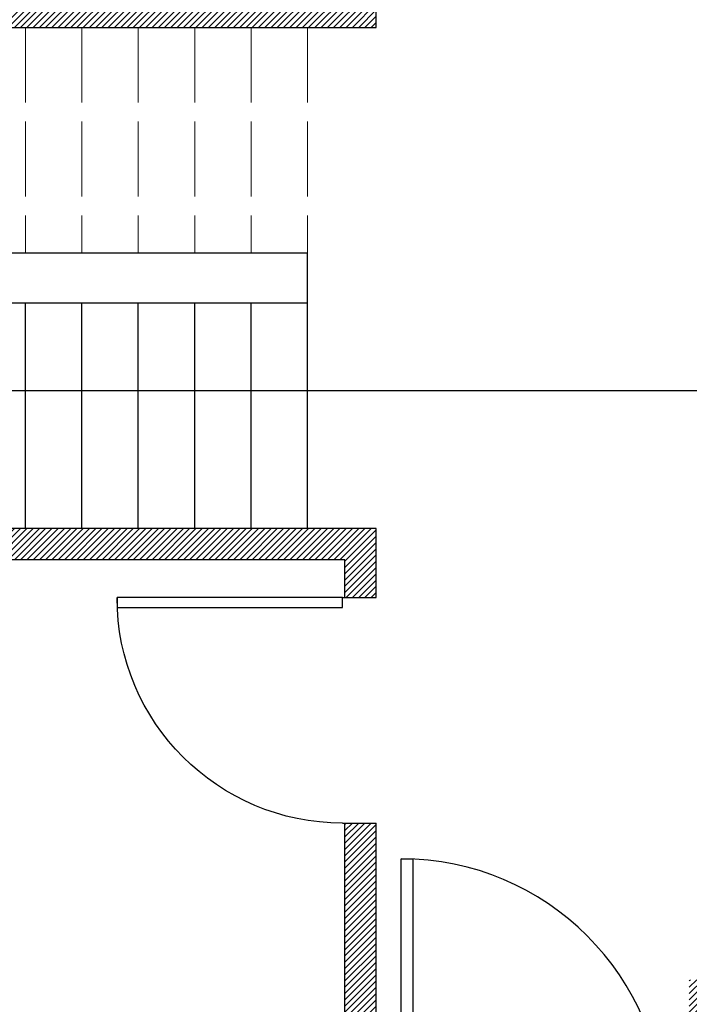
# Model space of a CAD drawing. Units: inches. Extents: x 2443635 to 2446153, y 1826255 to 1827341.
# Tile 3 of 16: x 2443784 to 2443891, y 1826991 to 1827149. Entities that reach past the tile are written whole.
import ezdxf

# ---------------------------------------------------------------- set-up
doc = ezdxf.new("R2010")
doc.units = ezdxf.units.IN
doc.linetypes.add('ACAD_ISO02W100', pattern=[15, 12, -3])
for name, color, linetype, lineweight in [('A-ANNO-SYMB', 4, 'Continuous', 25), ('A-DOOR', 2, 'Continuous', 25), ('A-STAIR', 7, 'Continuous', 25), ('A-STAIR-OVHD', 7, 'ACAD_ISO02W100', 18), ('A-WALL-INT', 9, 'Continuous', 30), ('A-WALL-PATT', 8, 'Continuous', 13)]:
    doc.layers.add(name, color=color, linetype=linetype, lineweight=lineweight)

# ---------------------------------------------------------------- blocks, each defined once
blk = doc.blocks.new('*U2')
for p, q in [((0, 0), (0, -6)), ((40, 0), (40, -6))]:
    blk.add_line(p, q)
blk.add_lwpolyline([(0, 0), (0, 40), (1.75, 40), (1.75, 0)], close=True)
blk.add_arc((0, 0), 40, 0, 90)

msp = doc.modelspace()

# ---------------------------------------------------------------- hatches: boundary and pattern name
at = {"layer": 'A-WALL-PATT'}
h = msp.add_hatch(dxfattribs=at)
h.set_pattern_fill('GOST_GROUND', color=256)
h.paths.add_polyline_path([(2443848.09, 1826870.288), (2443841.09, 1826870.288), (2443836.09, 1826870.288), (2443794.09, 1826870.288), (2443794.09, 1826861.288), (2443848.09, 1826861.288)])
h.paths.add_polyline_path([(2443935.09, 1826870.288), (2443896.09, 1826870.288), (2443891.09, 1826870.288), (2443884.09, 1826870.288), (2443884.09, 1826861.288), (2443935.09, 1826861.288)])
h.paths.add_polyline_path([(2444031.09, 1826999.288), (2444022.09, 1826999.288), (2444022.09, 1826995.288), (2444022.09, 1826990.288), (2444022.09, 1826870.288), (2443983.09, 1826870.288), (2443983.09, 1826861.288), (2444031.09, 1826861.288)])
h.paths.add_polyline_path([(2443758.09, 1826870.288), (2443716.09, 1826870.288), (2443716.09, 1826925.457, -0.0618154), (2443716.09, 1826925.788), (2443716.09, 1826948.288), (2443707.09, 1826948.288), (2443707.09, 1826861.288), (2443758.09, 1826861.288)])
h.paths.add_polyline_path([(2443716.09, 1827062.288), (2443716.09, 1827067.288), (2443716.09, 1827147.288), (2443716.09, 1827152.288), (2443716.09, 1827194.288), (2443707.09, 1827194.288), (2443707.09, 1826984.288), (2443716.09, 1826984.288)])
h.paths.add_polyline_path([(2443716.09, 1827296.288), (2443836.09, 1827296.288), (2443841.09, 1827296.288), (2443860.09, 1827296.288), (2443860.09, 1827305.288), (2443707.09, 1827305.288), (2443707.09, 1827254.288), (2443716.09, 1827254.288)])
h.paths.add_polyline_path([(2444031.09, 1827305.288), (2443878.09, 1827305.288), (2443878.09, 1827296.288), (2443881.588, 1827296.288), (2443897.09, 1827296.288), (2443902.09, 1827296.288), (2444022.09, 1827296.288), (2444022.09, 1827284.209), (2444022.09, 1827254.288), (2444031.09, 1827254.288)])
h.paths.add_polyline_path([(2444031.09, 1827194.288), (2444022.09, 1827194.288), (2444022.09, 1827152.288), (2444022.09, 1827147.288), (2444022.09, 1827113.953), (2444022.096, 1827113.948), (2444022.084, 1827080.628), (2444022.09, 1827047.288), (2444031.09, 1827047.288)])
h = msp.add_hatch(dxfattribs=at)
h.set_pattern_fill('JIS_WOOD', color=256)
h.paths.add_polyline_path([(2443841.09, 1827296.288), (2443836.09, 1827296.288), (2443836.09, 1827192.288), (2443841.09, 1827192.288), (2443841.09, 1827195.288), (2443861.09, 1827195.288), (2443861.09, 1827200.288), (2443841.09, 1827200.288)])
h.paths.add_polyline_path([(2443902.09, 1827296.288), (2443897.09, 1827296.288), (2443897.09, 1827200.288), (2443891.09, 1827200.288), (2443891.09, 1827195.288), (2443897.09, 1827195.288), (2443897.09, 1827192.288), (2443902.09, 1827192.288)])
h.paths.add_polyline_path([(2444022.09, 1827147.288), (2444022.09, 1827152.288), (2443902.09, 1827152.288), (2443902.09, 1827156.288), (2443897.09, 1827156.288), (2443897.09, 1827147.288)])
h.paths.add_polyline_path([(2443716.09, 1827152.288), (2443716.09, 1827147.288), (2443841.09, 1827147.288), (2443841.09, 1827156.288), (2443836.09, 1827156.288), (2443836.09, 1827152.288)])
h.paths.add_polyline_path([(2443836.09, 1827062.288), (2443836.09, 1827056.288), (2443841.09, 1827056.288), (2443841.09, 1827067.288), (2443716.09, 1827067.288), (2443716.09, 1827062.288)])
h.paths.add_polyline_path([(2443841.09, 1827020.288), (2443836.09, 1827020.288), (2443836.09, 1826870.288), (2443841.09, 1826870.288), (2443841.09, 1826966.288), (2443841.09, 1826971.288)])
h.paths.add_polyline_path([(2443896.09, 1826990.288), (2443980.09, 1826990.288), (2443980.09, 1826995.288), (2443891.09, 1826995.288), (2443891.09, 1826971.288), (2443891.09, 1826966.288), (2443891.09, 1826870.288), (2443896.09, 1826870.288)])

# ---------------------------------------------------------------- linework, layer by layer
at = {"layer": 'A-ANNO-SYMB'}
msp.add_line((2444060.214, 1827089.288), (2443676.359, 1827089.288), dxfattribs=at)
at = {"layer": 'A-STAIR'}
for p, q in [((2443752.09, 1827111.288), (2443830.09, 1827111.288)), ((2443830.09, 1827103.288), (2443830.09, 1827111.288)), ((2443830.09, 1827103.288), (2443752.09, 1827103.288)), ((2443785.09, 1827067.288), (2443785.09, 1827103.288)), ((2443794.09, 1827067.288), (2443794.09, 1827103.288)), ((2443803.09, 1827067.288), (2443803.09, 1827103.288)), ((2443812.09, 1827067.288), (2443812.09, 1827103.288)), ((2443821.09, 1827067.288), (2443821.09, 1827103.288)), ((2443830.09, 1827067.288), (2443830.09, 1827103.288))]:
    msp.add_line(p, q, dxfattribs=at)
at = {"layer": 'A-STAIR-OVHD'}
for p, q in [((2443785.09, 1827147.288), (2443785.09, 1827111.288)), ((2443794.09, 1827147.288), (2443794.09, 1827111.288)), ((2443803.09, 1827147.288), (2443803.09, 1827111.288)), ((2443812.09, 1827147.288), (2443812.09, 1827111.288)), ((2443821.09, 1827147.288), (2443821.09, 1827111.288)), ((2443830.09, 1827147.288), (2443830.09, 1827111.288))]:
    msp.add_line(p, q, dxfattribs=at)
at = {"layer": 'A-WALL-INT'}
for p, q in [((2443841.09, 1827147.288), (2443841.09, 1827156.288)), ((2443716.09, 1827147.288), (2443841.09, 1827147.288)), ((2443841.09, 1827067.288), (2443716.09, 1827067.288)), ((2443841.09, 1827056.288), (2443841.09, 1827067.288)), ((2443836.09, 1827062.288), (2443716.09, 1827062.288)), ((2443836.09, 1827056.288), (2443836.09, 1827062.288)), ((2443836.09, 1827056.288), (2443841.09, 1827056.288)), ((2443836.09, 1826870.288), (2443836.09, 1827020.288)), ((2443836.09, 1827020.288), (2443841.09, 1827020.288)), ((2443841.09, 1826971.288), (2443841.09, 1827020.288))]:
    msp.add_line(p, q, dxfattribs=at)

# ---------------------------------------------------------------- block references
at = {"layer": 'A-DOOR', "xscale": -0.9, "yscale": 0.9, "zscale": 0.9, "rotation": 90}
msp.add_blockref('*U2', (2443835.69, 1827056.288), dxfattribs=at)
at = {"layer": 'A-DOOR', "xscale": 1.05, "yscale": 1.05, "zscale": 1.05}
msp.add_blockref('*U2', (2443845.09, 1826972.588), dxfattribs=at)

doc.saveas('drawing.dxf')
